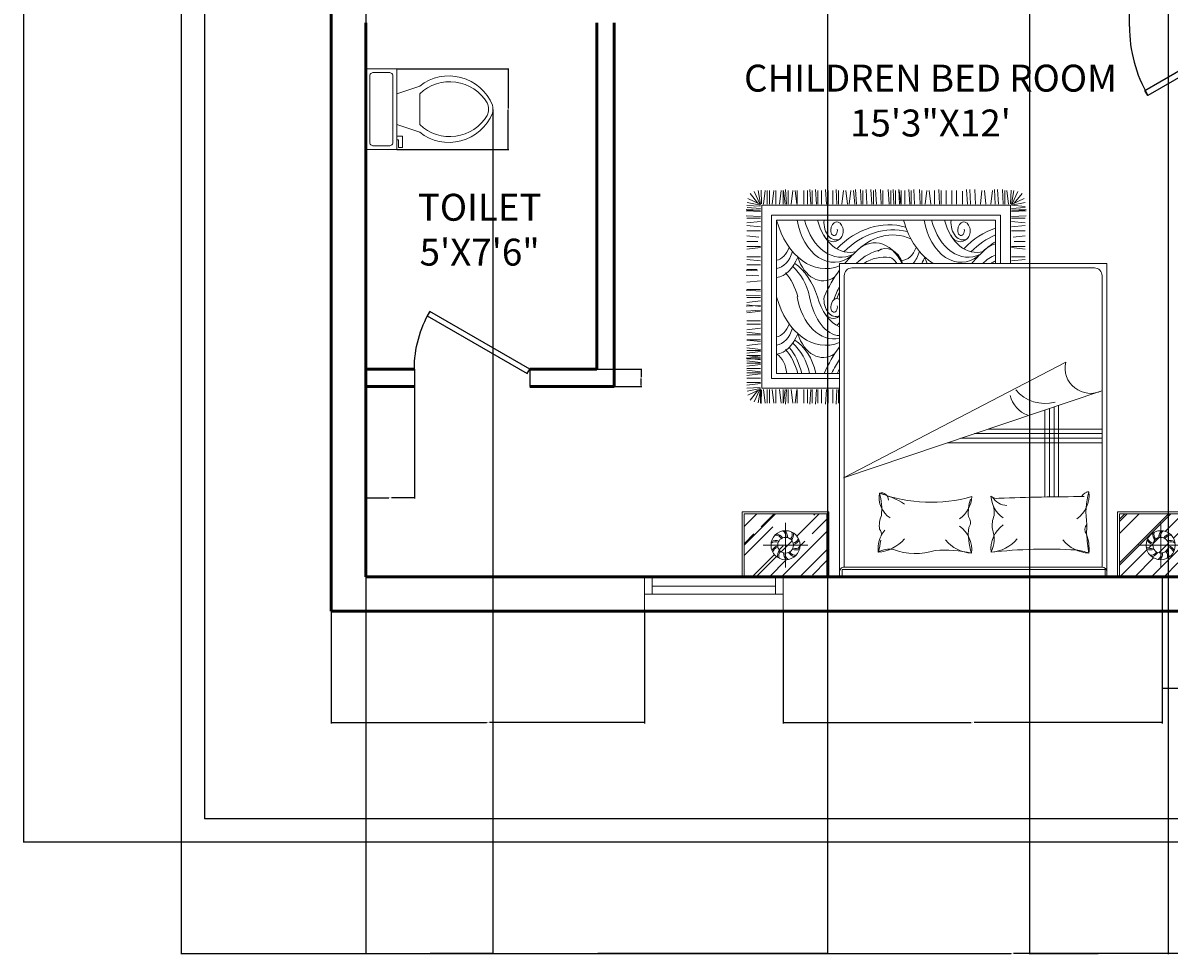
# Model space of a CAD drawing. Units: inches. Extents: x -28 to 483, y -584 to 51.
# Tile 1 of 6: x -28 to 270, y -584 to -342. Entities that reach past the tile are written whole.
import ezdxf

# ---------------------------------------------------------------- set-up
doc = ezdxf.new("R2010")
doc.units = ezdxf.units.IN
doc.header["$MEASUREMENT"] = 0
for name, color, linetype, lineweight in [('A-ANNO-DIMS', 2, 'Continuous', 18), ('A-AREA-IDEN', 7, 'Continuous', 25), ('A-DOOR', 4, 'Continuous', 25), ('A-FLOR-FIXT', 9, 'Continuous', 18), ('A-FURN', 30, 'Continuous', 18), ('A-GLAZ', 5, 'Continuous', 18), ('A-WALL', 7, 'Continuous', 50), ('C-PROP', 7, 'Continuous', 25)]:
    doc.layers.add(name, color=color, linetype=linetype, lineweight=lineweight)
doc.styles.get("Standard").update_dxf_attribs({"font": 'arial.ttf'})
doc.dimstyles.get("Standard").update_dxf_attribs({"dimtxt": 0.18, "dimasz": 0.18, "dimexe": 0.18, "dimexo": 0.0625, "dimgap": 0.09, "dimtad": 0, "dimtih": 1, "dimtoh": 1, "dimdec": 4, "dimzin": 0, "dimdsep": 46, "dimtxsty": 'Standard', "dimcen": 0.09, "dimadec": 0, "dimazin": 0, "dimtfac": 1, "dimtdec": 4, "dimtofl": 0, "dimtmove": 0, "dimatfit": 3, "dimfxl": 1, "dimtolj": 1, "dimtzin": 0, "dimarcsym": 0})

# ---------------------------------------------------------------- blocks, each defined once
blk = doc.blocks.new('*U2')
for p, q in [((0, 0), (0, -6)), ((40, 0), (40, -6))]:
    blk.add_line(p, q)
blk.add_lwpolyline([(0, 0), (34.64, 20), (35.52, 18.48), (0.87, -1.52)], close=True)
blk.add_arc((0, 0), 40, 0, 30)
blk = doc.blocks.new('A$C64B41DC1')
for p, q in [((0, 2.5079), (2.9903, 2.5079)), ((0, 2.0879), (0, 2.5079)), ((0.012, 2.4618), (0.0581, 2.5079)), ((0.012, 2.3515), (0.1684, 2.5079)), ((0.012, 2.0999), (0.012, 2.5079)), ((0.0543, 2.2213), (0.3409, 2.5079)), ((0.1689, 2.4179), (0.2589, 2.5079)), ((0.3265, 2.386), (0.4484, 2.5079)), ((0.3699, 2.3332), (0.5445, 2.5079)), ((0.548, 2.5079), (0.548, 2.0999)), ((0.56, 2.5079), (0.56, 2.0879)), ((0.6301, 2.5079), (0.6301, 0.4779)), ((0.6401, 2.461), (0.6401, 2.5079)), ((0.6401, 2.5079), (2.344, 2.5079)), ((2.344, 2.461), (0.6401, 2.461)), ((2.344, 2.5079), (2.3601, 2.5079)), ((2.344, 2.5079), (2.344, 2.461)), ((2.3601, 2.5079), (2.3601, 2.4761)), ((2.3601, 0.4779), (2.3601, 2.5079)), ((2.4303, 2.5079), (2.4303, 2.0879)), ((2.4423, 2.5079), (2.4423, 2.0999)), ((2.4423, 2.3333), (2.6169, 2.5079)), ((2.4423, 2.2145), (2.7357, 2.5079)), ((2.4423, 2.404), (2.5354, 2.4971)), ((2.705, 2.398), (2.8149, 2.5079)), ((2.7691, 2.3772), (2.8998, 2.5079)), ((2.7819, 2.3646), (2.9252, 2.5079)), ((2.9783, 2.0999), (2.9783, 2.5079)), ((2.9903, 2.0879), (2.9903, 2.5079)), ((0.2157, 2.0999), (0.548, 2.4322)), ((0.2299, 2.0999), (0.548, 2.418)), ((0.2804, 2.1597), (0.2804, 2.4481)), ((0.6601, 2.4461), (1.4951, 2.4461)), ((0.6601, 2.4461), (0.6601, 0.5579)), ((1.4951, 2.4461), (0.6697, 2.4461)), ((2.3301, 2.4461), (1.4951, 2.4461)), ((2.3301, 0.5579), (2.3301, 2.4461)), ((2.7099, 2.1597), (2.7099, 2.4481)), ((0.1362, 2.3039), (0.4246, 2.3039)), ((0.2311, 2.2906), (0.2937, 2.3532)), ((0.3405, 2.3039), (0.3605, 2.3238)), ((2.8541, 2.3039), (2.5657, 2.3039)), ((2.5849, 2.2779), (2.6158, 2.3088)), ((2.6158, 2.3088), (2.6313, 2.3243)), ((2.6674, 2.2756), (2.7382, 2.3464)), ((2.7249, 2.3076), (2.7512, 2.3339)), ((2.7746, 2.0999), (2.9783, 2.3036)), ((2.7914, 2.1846), (2.9783, 2.3715)), ((0.012, 2.261), (0.0275, 2.2765)), ((0.0404, 2.0999), (0.1982, 2.2578)), ((0.2905, 2.2539), (0.3304, 2.2938)), ((0.4194, 2.0999), (0.548, 2.2285)), ((2.4423, 2.1353), (2.5382, 2.2312)), ((2.4918, 2.0999), (2.6366, 2.2447)), ((2.9144, 2.2312), (2.9783, 2.2951)), ((0.1365, 2.0999), (0.251, 2.2144)), ((2.7831, 2.0999), (2.8678, 2.1846)), ((2.8962, 2.0999), (2.9783, 2.182)), ((0.56, 2.0879), (0, 2.0879)), ((0.548, 2.0999), (0.012, 2.0999)), ((0.4986, 2.0999), (0.548, 2.1493)), ((0.5127, 2.0999), (0.548, 2.1352)), ((2.4303, 2.0879), (2.9903, 2.0879)), ((2.4423, 2.0999), (2.9783, 2.0999)), ((2.5172, 2.0999), (2.5269, 2.1096)), ((0.9415, 1.9902), (0.9415, 1.3975)), ((0.9715, 1.9906), (0.9715, 1.4076)), ((1.0015, 1.991), (1.0015, 1.4177)), ((1.0315, 1.9916), (1.0315, 1.4279)), ((2.3349, 1.8678), (0.6613, 1.3029)), ((0.8956, 1.1191), (2.3349, 1.8678)), ((1.6636, 1.6412), (0.6601, 1.6412)), ((1.5748, 1.6112), (0.6601, 1.6112)), ((2.3665, 1.295), (2.3665, 1.3839)), ((2.377, 1.295), (2.3822, 1.3891)), ((2.4032, 1.295), (2.4032, 1.3839)), ((2.4346, 1.295), (2.4346, 1.3839)), ((2.4451, 1.295), (2.4503, 1.3891)), ((2.4774, 1.2957), (2.4774, 1.3837)), ((2.5, 1.295), (2.5, 1.3839)), ((2.5105, 1.295), (2.5157, 1.3891)), ((2.5367, 1.295), (2.5367, 1.3839)), ((2.5471, 1.295), (2.5524, 1.3891)), ((2.5681, 1.295), (2.5681, 1.3839)), ((2.5918, 1.295), (2.5918, 1.3839)), ((2.6346, 1.2957), (2.6346, 1.3837)), ((2.6362, 1.2957), (2.6467, 1.3839)), ((2.6729, 1.295), (2.6624, 1.3839)), ((2.6938, 1.295), (2.6938, 1.3839)), ((2.7043, 1.295), (2.7095, 1.3891)), ((2.7127, 1.2957), (2.7232, 1.3839)), ((2.7253, 1.295), (2.7253, 1.3839)), ((2.7494, 1.295), (2.7389, 1.3839)), ((2.7718, 1.295), (2.7718, 1.3839)), ((2.7959, 1.295), (2.7854, 1.3839)), ((2.8146, 1.2957), (2.8146, 1.3837)), ((2.8146, 1.2957), (2.8146, 1.3837)), ((2.8282, 1.295), (2.8282, 1.3839)), ((2.8282, 1.295), (2.8282, 1.3839)), ((2.8523, 1.295), (2.8418, 1.3839)), ((2.8523, 1.295), (2.8418, 1.3839)), ((2.8653, 1.2966), (2.8688, 1.3861)), ((2.8711, 1.2957), (2.8711, 1.3837)), ((2.8711, 1.2957), (2.8875, 1.3822)), ((2.8765, 1.2958), (2.9132, 1.3758)), ((2.8893, 1.3011), (2.9394, 1.3636)), ((2.3601, 1.2873), (2.8639, 1.2873)), ((2.8639, 1.2873), (2.8639, 0.1018)), ((2.8713, 1.2927), (2.954, 1.3315)), ((2.8716, 1.2565), (2.9605, 1.2669)), ((2.8717, 1.2884), (2.9588, 1.3058)), ((2.8744, 1.2817), (2.9603, 1.2869)), ((2.3601, 1.2233), (2.7999, 1.2233)), ((2.3601, 1.1913), (2.7679, 1.1912)), ((2.7679, 1.1912), (2.7679, 0.1978)), ((2.7999, 1.2233), (2.7999, 0.1658)), ((2.8716, 1.2212), (2.9605, 1.2212)), ((2.8716, 1.1947), (2.9605, 1.2052)), ((2.8723, 1.2489), (2.9603, 1.2489)), ((2.8716, 1.181), (2.9605, 1.1705)), ((2.8716, 1.1595), (2.9605, 1.1595)), ((2.8716, 1.133), (2.9605, 1.1435)), ((2.8716, 1.1193), (2.9605, 1.1088)), ((2.8723, 1.1872), (2.9603, 1.1872)), ((2.8723, 1.1255), (2.9603, 1.1255)), ((2.8716, 1.1035), (2.9605, 1.093)), ((2.8716, 1.0965), (2.9605, 1.0965)), ((2.8716, 1.086), (2.9657, 1.0913)), ((2.8716, 1.0756), (2.9605, 1.0756)), ((2.8716, 1.0491), (2.9605, 1.0596)), ((2.8723, 1.0858), (2.9605, 1.0753)), ((2.8723, 1.0416), (2.9603, 1.0416)), ((2.8716, 1.0354), (2.9605, 1.0249)), ((2.8723, 0.9987), (2.9605, 1.0092)), ((2.8723, 0.985), (2.9605, 0.9745)), ((2.8723, 0.9735), (2.9603, 0.9735)), ((2.8716, 0.9346), (2.9605, 0.9241)), ((2.8723, 0.9408), (2.9603, 0.9408)), ((2.8723, 0.8979), (2.9605, 0.9084)), ((2.8723, 0.8726), (2.9603, 0.8726)), ((2.8723, 0.8505), (2.9603, 0.8505)), ((2.8716, 0.7885), (2.9605, 0.799)), ((2.8716, 0.7818), (2.9657, 0.787)), ((2.8716, 0.7503), (2.9657, 0.7556)), ((2.8723, 0.7571), (2.9605, 0.7466)), ((2.8716, 0.7204), (2.9605, 0.7309)), ((2.8716, 0.6995), (2.9605, 0.6995)), ((2.8716, 0.689), (2.9657, 0.6838)), ((2.8716, 0.6576), (2.9657, 0.6523)), ((2.8716, 0.6471), (2.9605, 0.6471)), ((2.8716, 0.5903), (2.9605, 0.6007)), ((2.882, 0.5582), (2.9657, 0.5536)), ((2.8909, 0.5263), (2.9657, 0.5222)), ((0.6301, 0.4779), (2.3601, 0.4779)), ((0.7101, 0.5079), (2.2801, 0.5079)), ((1.2465, 0.4625), (1.1576, 0.452)), ((1.2542, 0.1018), (1.2542, 0.4779)), ((1.3182, 0.1658), (1.3182, 0.4779)), ((1.3502, 0.1978), (1.3502, 0.4779)), ((2.8716, 0.4877), (2.9603, 0.4877)), ((2.8716, 0.4625), (2.9605, 0.452)), ((2.8928, 0.5169), (2.9605, 0.5169)), ((1.2465, 0.3746), (1.1576, 0.3851)), ((1.2465, 0.4365), (1.1577, 0.4365)), ((2.8716, 0.4365), (2.9603, 0.4365)), ((2.8716, 0.3746), (2.9605, 0.3851)), ((1.2355, 0.3092), (1.1576, 0.3)), ((1.2465, 0.3684), (1.1577, 0.3684)), ((1.2285, 0.3357), (1.1577, 0.3357)), ((2.8716, 0.3684), (2.9603, 0.3684)), ((2.8826, 0.3092), (2.9605, 0.3)), ((2.8896, 0.3357), (2.9603, 0.3357)), ((1.2457, 0.2423), (1.1576, 0.2319)), ((1.2457, 0.2676), (1.1577, 0.2676)), ((2.8723, 0.2676), (2.9603, 0.2676)), ((2.8723, 0.2423), (2.9605, 0.2319)), ((1.2465, 0.1742), (1.1524, 0.169)), ((1.2465, 0.2057), (1.1576, 0.2161)), ((1.2465, 0.1847), (1.1576, 0.1847)), ((2.7999, 0.1658), (1.3182, 0.1658)), ((2.7679, 0.1978), (1.3502, 0.1978)), ((2.8716, 0.2057), (2.9605, 0.2161)), ((2.8716, 0.1847), (2.9605, 0.1847)), ((2.8716, 0.1742), (2.9657, 0.169)), ((1.2465, 0.1428), (1.1524, 0.1376)), ((1.2465, 0.1334), (1.1524, 0.1281)), ((1.2465, 0.1323), (1.1576, 0.1323)), ((1.2465, 0.1323), (1.1576, 0.1323)), ((1.2465, 0.1), (1.1576, 0.1105)), ((1.2465, 0.1229), (1.1588, 0.1168)), ((1.2464, 0.1007), (1.1592, 0.0833)), ((1.2468, 0.0964), (1.1641, 0.0576)), ((1.2288, 0.088), (1.1787, 0.0255)), ((1.2415, 0.0933), (1.2049, 0.0133)), ((1.247, 0.0934), (1.2306, 0.0069)), ((1.2527, 0.0925), (1.2493, 0.003)), ((2.8639, 0.1018), (1.2542, 0.1018)), ((1.2658, 0.0941), (1.2762, 0.0052)), ((1.2899, 0.0941), (1.2899, 0.0052)), ((1.2999, 0.0941), (1.3051, 0)), ((1.3313, 0.0941), (1.3365, 0)), ((1.3523, 0.0941), (1.3575, 0)), ((1.3804, 0.0941), (1.3699, 0.0052)), ((1.4119, 0.0934), (1.4223, 0.0052)), ((1.4485, 0.0941), (1.438, 0.0052)), ((1.48, 0.0941), (1.4852, 0)), ((1.5114, 0.0941), (1.5166, 0)), ((1.5323, 0.0941), (1.5376, 0)), ((1.5638, 0.0941), (1.5638, 0.0105)), ((1.6021, 0.0941), (1.6021, 0.0052)), ((1.6336, 0.0941), (1.6336, 0.0052)), ((1.6702, 0.0941), (1.6702, 0.0052)), ((1.7017, 0.0941), (1.7017, 0.0052)), ((1.7122, 0.0941), (1.7174, 0)), ((1.7445, 0.0934), (1.7445, 0.0054)), ((1.7698, 0.0934), (1.7803, 0.0052)), ((1.8065, 0.0941), (1.796, 0.0052)), ((1.8274, 0.0941), (1.8274, 0.0052)), ((1.8379, 0.0941), (1.8431, 0)), ((1.8746, 0.0941), (1.8798, 0)), ((1.8955, 0.0941), (1.8955, 0.0052)), ((1.906, 0.0941), (1.9113, 0)), ((1.9384, 0.0934), (1.9384, 0.0054)), ((1.9609, 0.0941), (1.9609, 0.0052)), ((1.9636, 0.0934), (1.9741, 0.0052)), ((1.9714, 0.0941), (1.9766, 0)), ((1.9976, 0.0941), (1.9976, 0.0052)), ((2.0081, 0.0941), (2.0133, 0)), ((2.029, 0.0941), (2.029, 0.0052)), ((2.0395, 0.0941), (2.0447, 0)), ((2.0797, 0.0941), (2.0797, 0.0052)), ((2.0902, 0.0941), (2.0954, 0)), ((2.1216, 0.0941), (2.1269, 0)), ((2.1412, 0.0941), (2.1412, 0.0052)), ((2.1517, 0.0941), (2.1569, 0)), ((2.1831, 0.0941), (2.1884, 0)), ((2.2093, 0.0941), (2.2093, 0.0052)), ((2.2198, 0.0941), (2.225, 0)), ((2.2512, 0.0941), (2.2565, 0)), ((2.2603, 0.0934), (2.2707, 0.0052)), ((2.2969, 0.0941), (2.2864, 0.0052)), ((2.3089, 0.0934), (2.3193, 0.0052)), ((2.3455, 0.0941), (2.3351, 0.0052)), ((2.3665, 0.0941), (2.3665, 0.0052)), ((2.377, 0.0941), (2.3822, 0)), ((2.4032, 0.0941), (2.4032, 0.0052)), ((2.4346, 0.0941), (2.4346, 0.0052)), ((2.4451, 0.0941), (2.4503, 0)), ((2.4774, 0.0934), (2.4774, 0.0054)), ((2.5, 0.0941), (2.5, 0.0052)), ((2.5105, 0.0941), (2.5157, 0)), ((2.5367, 0.0941), (2.5367, 0.0052)), ((2.5471, 0.0941), (2.5524, 0)), ((2.5681, 0.0941), (2.5681, 0.0052)), ((2.5918, 0.0941), (2.5918, 0.0052)), ((2.6346, 0.0934), (2.6346, 0.0054)), ((2.6362, 0.0934), (2.6467, 0.0052)), ((2.6729, 0.0941), (2.6624, 0.0052)), ((2.6938, 0.0941), (2.6938, 0.0052)), ((2.7043, 0.0941), (2.7095, 0)), ((2.7127, 0.0934), (2.7232, 0.0052)), ((2.7253, 0.0941), (2.7253, 0.0052)), ((2.7494, 0.0941), (2.7389, 0.0052)), ((2.7718, 0.0941), (2.7718, 0.0052)), ((2.7959, 0.0941), (2.7854, 0.0052)), ((2.8146, 0.0934), (2.8146, 0.0054)), ((2.8282, 0.0941), (2.8282, 0.0052)), ((2.8523, 0.0941), (2.8418, 0.0052)), ((2.8653, 0.0925), (2.8688, 0.003)), ((2.8711, 0.0934), (2.8875, 0.0069)), ((2.8713, 0.0964), (2.954, 0.0576)), ((2.8716, 0.1428), (2.9657, 0.1376)), ((2.8716, 0.1334), (2.9657, 0.1281)), ((2.8716, 0.1323), (2.9605, 0.1323)), ((2.8716, 0.1229), (2.9593, 0.1168)), ((2.8717, 0.1007), (2.9588, 0.0833)), ((2.8744, 0.1074), (2.9603, 0.1022)), ((2.8765, 0.0933), (2.9132, 0.0133)), ((2.8893, 0.088), (2.9394, 0.0255))]:
    blk.add_line(p, q)
at = {"ltscale": 10}
for p, q in [((1.4859, 1.5812), (0.6601, 1.5812)), ((1.397, 1.5512), (0.6601, 1.5512))]:
    blk.add_line(p, q, dxfattribs=at)
for centre, radius in [((0.2804, 2.3039), 0.0942), ((2.7099, 2.3039), 0.0942), ((0.2804, 2.3039), 0.051), ((2.7099, 2.3039), 0.051)]:
    blk.add_circle(centre, radius)
for centre, radius, start, end in [((0.6601, 2.4761), 0.03, 180, 270), ((2.3301, 2.4761), 0.03, 270, 0), ((0.2887, 2.3745), 0.0605, 172.17003, 218.48975), ((0.2828, 2.3731), 0.0462, 160.30017, 220.53802), ((0.3286, 2.3561), 0.0605, 136.17003, 182.48975), ((0.3231, 2.3585), 0.0462, 124.30017, 184.53802), ((0.3501, 2.3178), 0.0605, 100.17003, 146.48975), ((2.6402, 2.3178), 0.0605, 33.51025, 79.82997), ((2.6672, 2.3585), 0.0462, 355.46198, 55.69983), ((2.6617, 2.3561), 0.0605, 357.51025, 43.82997), ((2.7075, 2.3731), 0.0462, 319.46198, 19.69983), ((2.7016, 2.3745), 0.0605, 321.51025, 7.82997), ((0.2457, 2.3659), 0.0605, 208.17003, 254.48975), ((0.2417, 2.3614), 0.0462, 196.30017, 256.53802), ((0.347, 2.323), 0.0462, 88.30017, 148.53802), ((0.3449, 2.2742), 0.0605, 64.17003, 110.48975), ((0.3455, 2.2802), 0.0462, 52.30017, 112.53802), ((1.0526, 2.3302), 0.3085, 175.30484, 198.69419), ((-0.8702, 2.0941), 1.6364, 4.80985, 9.18918), ((0.8579, 2.6278), 0.2948, 247.51785, 264.26696), ((0.728, 2.111), 0.245, 40.4189, 85.9871), ((1.0164, 5.7096), 3.3803, 266.81337, 276.16021), ((1.3963, 2.1044), 0.245, 94.0129, 139.5811), ((1.1858, 2.3288), 0.1943, 306.5711, 5.88998), ((1.5348, 2.2652), 0.1767, 151.77364, 201.69827), ((1.6986, 2.3355), 0.1943, 174.11002, 233.4289), ((1.1481, 2.2311), 0.3783, 353.49469, 19.18669), ((1.6871, 3.192), 0.8561, 257.74383, 273.62843), ((1.4882, 2.111), 0.245, 40.4189, 85.9871), ((1.8674, 1.9709), 0.3878, 68.20259, 108.9817), ((2.1269, 2.1044), 0.245, 94.0129, 139.5811), ((2.0342, 2.4856), 0.1563, 261.59582, 298.90918), ((1.9165, 2.3288), 0.1943, 333.73715, 5.88998), ((2.6058, 2.2028), 0.517, 163.60457, 172.3273), ((2.6448, 2.2802), 0.0462, 67.46198, 127.69983), ((2.6454, 2.2742), 0.0605, 69.51025, 115.82997), ((2.6433, 2.323), 0.0462, 31.46198, 91.69983), ((2.7486, 2.3614), 0.0462, 283.46198, 343.69983), ((2.7446, 2.3659), 0.0605, 285.51025, 331.82997), ((0.2153, 2.3276), 0.0462, 232.30017, 292.53802), ((0.2158, 2.3336), 0.0605, 244.17003, 290.48975), ((0.2138, 2.2848), 0.0462, 268.30017, 328.53802), ((0.2107, 2.29), 0.0605, 280.17003, 326.48975), ((0.2377, 2.2493), 0.0462, 304.30017, 4.53802), ((0.2322, 2.2517), 0.0605, 316.17003, 2.48975), ((0.2779, 2.2347), 0.0462, 340.30017, 40.53802), ((0.272, 2.2333), 0.0605, 352.17003, 38.48975), ((0.3191, 2.2464), 0.0462, 16.30017, 76.53802), ((0.3151, 2.2419), 0.0605, 28.17003, 74.48975), ((0.7274, 2.2013), 0.0446, 314.4736, 42.17134), ((-1.6008, 2.277), 2.3618, 357.39054, 358.88764), ((1.9165, 2.3288), 0.1943, 320.94042, 333.73715), ((2.1347, 2.2313), 0.0459, 165.35061, 223.26844), ((2.6752, 2.2419), 0.0605, 105.51025, 151.82997), ((2.6712, 2.2464), 0.0462, 103.46198, 163.69983), ((2.7182, 2.2333), 0.0605, 141.51025, 187.82997), ((2.7123, 2.2347), 0.0462, 139.46198, 199.69983), ((2.7581, 2.2517), 0.0605, 177.51025, 223.82997), ((2.7526, 2.2493), 0.0462, 175.46198, 235.69983), ((2.7796, 2.29), 0.0605, 213.51025, 259.82997), ((2.7765, 2.2848), 0.0462, 211.46198, 271.69983), ((2.7744, 2.3336), 0.0605, 249.51025, 295.82997), ((2.775, 2.3276), 0.0462, 247.46198, 307.69983), ((0.2688, 2.0945), 0.4956, 344.0243, 8.70709), ((1.204, 2.1778), 0.1681, 337.01697, 7.53676), ((1.5671, 2.1546), 0.0547, 142.08329, 220.902), ((1.9346, 2.1778), 0.1681, 337.01697, 7.53676), ((0.9385, 1.978), 0.1943, 126.5711, 185.88998), ((1.1858, 1.9714), 0.1943, 4.31813, 53.4289), ((1.5415, 2.0969), 0.1834, 175.22328, 196.23004), ((1.7059, 1.9714), 0.204, 127.11975, 175.09005), ((1.1965, 2.0983), 0.3299, 343.79543, 3.55541), ((1.9394, 1.991), 0.1651, 351.26213, 55.75721), ((2.4617, 2.0719), 0.3745, 173.82958, 196.4356), ((1.2687, 1.9248), 0.1223, 33.62799, 86.47438), ((1.7676, 1.0629), 0.9631, 69.65065, 105.96307), ((2.2748, 2.5795), 0.6373, 238.34989, 254.31375), ((2.0911, 2.0123), 0.0478, 179.77267, 283.80184), ((0.7417, 2.0149), 0.057, 273.47085, 328.54118), ((0.728, 2.2025), 0.245, 274.0129, 278.34166), ((0.7246, 18.8439), 16.8552, 270.17399, 272.05214), ((1.3401, 1.9404), 0.0603, 49.09906, 101.37023), ((1.0747, 1.2871), 0.1871, 14.1863, 69.12121), ((1.0274, 1.1334), 0.2527, 40.62904, 104.37123), ((0.7347, 1.1553), 0.1649, 347.31088, 116.44537), ((0.7101, 0.5579), 0.05, 180, 270), ((2.2801, 0.5579), 0.05, 270, 0)]:
    blk.add_arc(centre, radius, start, end)
for centre, major_axis, ratio, start_param, end_param in [((1.9938, 1.6262), (0, -0.7531), 0.68, 0.797284, 0.954936), ((2.0643, 1.466), (0, -0.5322), 0.68, 7.239912, 7.311536), ((1.9052, 1.7397), (0, -0.9842), 0.68, 0.74745, 0.979724), ((2.7455, 1.3081), (0, 0.3614), 0.68, 1.900046, 2.742661), ((2.7868, 1.3081), (0, 0.3614), 0.68, 1.900046, 2.614747), ((2.8372, 1.3081), (0, 0.3614), 0.68, 1.900046, 2.479658), ((2.8607, 1.3211), (0, 0.3614), 0.68, 1.938265, 2.479658), ((2.8057, 1.2079), (0, -0.1524), 0.68, 4.821745, 5.895886), ((2.4665, 0.8216), (0, -0.2664), 0.68, 2.006169, 3.565187), ((2.4513, 0.5069), (0, 0.502), 0.68, 5.095327, 6.553458), ((2.7862, 0.8069), (0, -0.2615), 0.68, 3.244645, 4.205018), ((2.396, 0.6032), (0, 0.3641), 0.68, -1.3172, 0.145284), ((2.7784, 0.8289), (0, -0.1802), 0.68, 3.227058, 4.318474), ((2.3507, 0.5642), (0.0073, 0.3819), 0.56205, -1.21172, -0.009991), ((2.7821, 0.7971), (0, -0.1589), 0.68, 3.272942, 4.229533), ((2.2964, 0.5771), (0, -0.3263), 0.68, 1.938944, 2.850232), ((2.0403, 1.6015), (0, -0.8763), 0.68, 6.849801, 6.887077), ((2.4005, 0.7132), (0, -0.1214), 0.68, 2.284368, 3.652258), ((2.3834, 0.7081), (0, 0.1147), 0.68, 4.593909, 6.585576), ((2.3774, 0.7653), (0, -0.0593), 0.68, 5.841311, 7.755362), ((2.3961, 0.7628), (0, -0.0317), 0.68, 1.462497, 5.046281), ((1.9938, 1.1295), (-0.0678, 0.7439), 0.610498, 3.917146, 4.063997), ((2.0643, 0.9693), (0, -0.5322), 0.68, 7.239912, 7.336618), ((1.9052, 1.243), (0, -0.9842), 0.68, 0.74745, 0.979724), ((2.7455, 0.8114), (-0.0599, 0.3735), 0.695517, 1.775813, 2.548612), ((2.7868, 0.8114), (0, 0.3614), 0.68, 1.900046, 2.614747), ((2.8607, 0.8243), (0, 0.3614), 0.68, 1.938265, 2.479658), ((2.4665, 0.3249), (0, -0.2664), 0.68, 2.006169, 3.565187), ((2.4513, 0.0102), (0, 0.502), 0.68, 5.095327, 6.553458), ((2.7862, 0.3102), (0, -0.2615), 0.68, 3.244645, 4.205018), ((1.242, 0.9693), (0, -0.5322), 0.68, 6.586764, 6.677612), ((1.1714, 1.1295), (-0.1157, 0.7241), 0.59432, 3.291697, 3.50733), ((1.0828, 1.243), (0, -0.9842), 0.68, 0.565948, 0.680366), ((1.5283, 0.0674), (0, -0.3703), 0.68, 1.930561, 3.464283), ((1.5736, 0.1065), (0, 0.3641), 0.68, -1.3172, 0.476403), ((1.6289, 0.0102), (0, 0.502), 0.68, 6.655152, 6.661293), ((1.6289, 0.0102), (0, 0.502), 0.68, 5.095327, 5.911219), ((1.6442, 0.3249), (0, -0.2664), 0.68, 2.006169, 2.182797), ((1.9638, 0.3102), (0, -0.2615), 0.68, 4.015924, 4.205018), ((1.956, 0.3322), (0, -0.1802), 0.68, 3.770744, 4.318474), ((1.9597, 0.3004), (0, -0.1589), 0.68, 3.14258, 4.229533), ((2.0606, 0.5616), (0, -0.1803), 0.68, 5.194792, 5.929328), ((2.0606, 0.5616), (0, -0.1803), 0.68, 5.194792, 6.723255), ((2.1315, 0.6603), (0, -0.3155), 0.68, 5.328638, 6.949396), ((2.0549, 0.5656), (0, -0.1303), 0.68, 5.450951, 6.054641), ((2.0643, 0.9693), (0, -0.5322), 0.68, 6.20013, 6.677612), ((1.9938, 1.1295), (-0.0678, 0.7439), 0.610498, 3.199135, 3.592282), ((1.9052, 1.243), (0, -0.9842), 0.68, 0.565948, 0.680366), ((2.3507, 0.0674), (0, -0.3703), 0.68, 1.930561, 3.464283), ((2.396, 0.1065), (0, 0.3641), 0.68, -1.3172, 0.476403), ((2.4513, 0.0102), (0, 0.502), 0.68, 6.655152, 6.661293), ((2.7784, 0.3322), (0, -0.1802), 0.68, 3.227058, 4.318474), ((2.7821, 0.3004), (0, -0.1589), 0.68, 3.272942, 4.229533), ((1.1933, 0.9181), (0, -0.624), 0.68, 0.378672, 0.625379), ((1.3091, 0.6603), (0, -0.3155), 0.68, 6.475719, 6.949396), ((1.1911, 1.1066), (0, 0.8458), 0.68, 3.421828, 3.728616), ((1.2179, 1.1047), (0, -0.8763), 0.68, 6.507006, 6.887077), ((1.474, 0.0804), (0, -0.3263), 0.68, 1.938944, 3.339184), ((2.0157, 0.9181), (0, -0.624), 0.68, -0.280078, 0.625379), ((2.0135, 1.1066), (0, 0.8458), 0.68, 2.978727, 3.728616), ((2.0403, 1.1047), (0, -0.8763), 0.68, 6.099302, 6.887077), ((2.2964, 0.0804), (0, -0.3263), 0.68, 1.938944, 3.339184), ((1.555, 0.2685), (0, -0.0593), 0.68, 3.732151, 7.755362), ((1.5781, 0.2165), (0, -0.1214), 0.68, 2.284368, 3.726131), ((1.561, 0.2114), (0, 0.1147), 0.68, 4.593909, 6.647252), ((1.5737, 0.2661), (0, -0.0317), 0.68, 1.462497, 5.046281), ((2.3774, 0.2685), (0, -0.0593), 0.68, 3.732151, 7.755362), ((2.4005, 0.2165), (0, -0.1214), 0.68, 2.284368, 3.726131), ((2.3834, 0.2114), (0, 0.1147), 0.68, 4.593909, 6.647252), ((2.3961, 0.2661), (0, -0.0317), 0.68, 1.462497, 5.046281)]:
    blk.add_ellipse(centre, major_axis=major_axis, ratio=ratio, start_param=start_param, end_param=end_param)
blk = doc.blocks.new('*U5')
for p, q in [((9.5, -6), (9.5, -2)), ((-10, -8.5), (-8, -8.5)), ((-10, -9.5), (-10, -8.5)), ((-8, -8.5), (-8, -8)), ((-7, -8), (-7, -9.5)), ((-4, -8), (-6, -14)), ((4, -8), (6, -14)), ((-7, -9.5), (-10, -9.5)), ((4, -14), (-4, -14))]:
    blk.add_line(p, q)
blk.add_lwpolyline([(10.5, -8), (10.5, 0), (-10.5, 0), (-10.5, -8)], close=True)
for points in [[(-9.5, -2), (-9.5, -6)], [(8.5, -1), (-8.5, -1)], [(-8.5, -7), (8.5, -7)]]:
    blk.add_lwpolyline(points)
for centre, radius, start, end in [((-8.62, -1.88), 0.884, 81.8699, 188.1301), ((8.62, -1.88), 0.884, 351.8699, 98.1301), ((-8.62, -6.12), 0.884, 171.8699, 278.1301), ((8.62, -6.12), 0.884, 261.8699, 8.1301), ((3.52, -21.58), 12.17, 141.4691, 247.9714), ((4.2, -21.82), 11.33, 136.3677, 238.9468), ((-3.52, -21.58), 12.17, 292.0284, 38.5307), ((-4.2, -21.82), 11.33, 301.053, 43.6321), ((0, -27.88), 4, 245.7318, 294.2682), ((0, -29), 4, 254.8605, 285.1395)]:
    blk.add_arc(centre, radius, start, end)
blk = doc.blocks.new('WIN-36IN')
for p, q in [((0, 9), (0, 0)), ((2, 9), (2, 4.5)), ((34, 9), (34, 4.5)), ((36, 9), (36, 0)), ((34, 6.5), (2, 6.5)), ((36, 4.5), (0, 4.5))]:
    blk.add_line(p, q)
blk = doc.blocks.new('*D19')
at = {"layer": 'A-ANNO-DIMS', "color": 0, "lineweight": -2, "transparency": 16777216}
for p, q in [((12.84, -554.65), (12.84, -583.72)), ((444.84, -554.65), (444.84, -583.72)), ((13.02, -583.54), (228.55, -583.54)), ((444.66, -583.54), (229.13, -583.54))]:
    blk.add_line(p, q, dxfattribs=at)
at = {"layer": 'A-ANNO-DIMS', "color": 0, "transparency": 16777216}
for points in [[(13.02, -583.51), (13.02, -583.57), (12.84, -583.54)], [(444.66, -583.51), (444.66, -583.57), (444.84, -583.54)]]:
    blk.add_solid(points, dxfattribs=at)
at = {"layer": 'Defpoints', "color": 0, "transparency": 16777216}
for p in [(12.84, -554.59), (444.84, -554.59), (444.84, -583.54)]:
    blk.add_point(p, dxfattribs=at)
at = {"layer": 'A-ANNO-DIMS', "color": 0, "transparency": 16777216, "insert": (228.84, -583.54), "char_height": 0.18, "attachment_point": 5}
blk.add_mtext('\\A1;432', dxfattribs=at)
blk = doc.blocks.new('*D20')
at = {"layer": 'A-ANNO-DIMS', "color": 0, "lineweight": -2, "transparency": 16777216}
for p, q in [((12.78, 21.41), (-28.29, 21.41)), ((-28.11, 21.23), (-28.11, -266.41)), ((-28.11, -554.41), (-28.11, -266.77)), ((12.78, -554.59), (-28.29, -554.59))]:
    blk.add_line(p, q, dxfattribs=at)
at = {"layer": 'A-ANNO-DIMS', "color": 0, "transparency": 16777216}
for points in [[(-28.14, 21.23), (-28.08, 21.23), (-28.11, 21.41)], [(-28.14, -554.41), (-28.08, -554.41), (-28.11, -554.59)]]:
    blk.add_solid(points, dxfattribs=at)
at = {"layer": 'Defpoints', "color": 0, "transparency": 16777216}
for p in [(-28.11, 21.41), (12.84, 21.41), (12.84, -554.59)]:
    blk.add_point(p, dxfattribs=at)
at = {"layer": 'A-ANNO-DIMS', "color": 0, "transparency": 16777216, "insert": (-28.11, -266.59), "char_height": 0.18, "attachment_point": 5}
blk.add_mtext('\\A1;576', dxfattribs=at)
blk = doc.blocks.new('*D26')
at = {"layer": 'A-ANNO-DIMS', "color": 0, "lineweight": -2, "transparency": 16777216}
for p, q in [((60.84, -337.15), (60.84, -583.72)), ((180.84, -337.15), (180.84, -583.72)), ((61.02, -583.54), (120.56, -583.54)), ((180.66, -583.54), (121.12, -583.54))]:
    blk.add_line(p, q, dxfattribs=at)
at = {"layer": 'A-ANNO-DIMS', "color": 0, "transparency": 16777216}
for points in [[(61.02, -583.51), (61.02, -583.57), (60.84, -583.54)], [(180.66, -583.51), (180.66, -583.57), (180.84, -583.54)]]:
    blk.add_solid(points, dxfattribs=at)
at = {"layer": 'Defpoints', "color": 0, "transparency": 16777216}
for p in [(60.84, -337.09), (180.84, -337.09), (180.84, -583.54)]:
    blk.add_point(p, dxfattribs=at)
at = {"layer": 'A-ANNO-DIMS', "color": 0, "transparency": 16777216, "insert": (120.84, -583.54), "char_height": 0.18, "attachment_point": 5}
blk.add_mtext('\\A1;120', dxfattribs=at)
blk = doc.blocks.new('*D28')
at = {"layer": 'A-ANNO-DIMS', "color": 0, "lineweight": -2, "transparency": 16777216}
for p, q in [((233.35, -193.15), (233.35, -583.72)), ((269.35, -193.15), (269.35, -583.72)), ((233.53, -583.54), (251.13, -583.54)), ((269.17, -583.54), (251.57, -583.54))]:
    blk.add_line(p, q, dxfattribs=at)
at = {"layer": 'A-ANNO-DIMS', "color": 0, "transparency": 16777216}
for points in [[(233.53, -583.51), (233.53, -583.57), (233.35, -583.54)], [(269.17, -583.51), (269.17, -583.57), (269.35, -583.54)]]:
    blk.add_solid(points, dxfattribs=at)
at = {"layer": 'Defpoints', "color": 0, "transparency": 16777216}
for p in [(233.35, -193.09), (269.35, -193.09), (269.35, -583.54)]:
    blk.add_point(p, dxfattribs=at)
at = {"layer": 'A-ANNO-DIMS', "color": 0, "transparency": 16777216, "insert": (251.35, -583.54), "char_height": 0.18, "attachment_point": 5}
blk.add_mtext('\\A1;36', dxfattribs=at)
blk = doc.blocks.new('*D36')
at = {"layer": 'A-ANNO-DIMS', "color": 0, "lineweight": -2, "transparency": 16777216}
for p, q in [((51.84, -494.65), (51.84, -523.72)), ((133.26, -494.65), (133.26, -523.72)), ((52.02, -523.54), (92.17, -523.54)), ((133.08, -523.54), (92.93, -523.54))]:
    blk.add_line(p, q, dxfattribs=at)
at = {"layer": 'A-ANNO-DIMS', "color": 0, "transparency": 16777216}
for points in [[(52.02, -523.51), (52.02, -523.57), (51.84, -523.54)], [(133.08, -523.51), (133.08, -523.57), (133.26, -523.54)]]:
    blk.add_solid(points, dxfattribs=at)
at = {"layer": 'Defpoints', "color": 0, "transparency": 16777216}
for p in [(51.84, -494.59), (133.26, -494.59), (51.84, -523.54)]:
    blk.add_point(p, dxfattribs=at)
at = {"layer": 'A-ANNO-DIMS', "color": 0, "transparency": 16777216, "insert": (92.55, -523.54), "char_height": 0.18, "attachment_point": 5}
blk.add_mtext('\\A1;81.41', dxfattribs=at)
blk = doc.blocks.new('*D39')
at = {"layer": 'A-ANNO-DIMS', "color": 0, "lineweight": -2, "transparency": 16777216}
for p, q in [((93.84, -364.08), (93.84, -583.72)), ((60.84, -374.58), (60.84, -583.72)), ((61.02, -583.54), (77.12, -583.54)), ((93.66, -583.54), (77.56, -583.54))]:
    blk.add_line(p, q, dxfattribs=at)
at = {"layer": 'A-ANNO-DIMS', "color": 0, "transparency": 16777216}
for points in [[(61.02, -583.51), (61.02, -583.57), (60.84, -583.54)], [(93.66, -583.51), (93.66, -583.57), (93.84, -583.54)]]:
    blk.add_solid(points, dxfattribs=at)
at = {"layer": 'Defpoints', "color": 0, "transparency": 16777216}
for p in [(93.84, -364.02), (60.84, -374.52), (93.84, -583.54)]:
    blk.add_point(p, dxfattribs=at)
at = {"layer": 'A-ANNO-DIMS', "color": 0, "transparency": 16777216, "insert": (77.34, -583.54), "char_height": 0.18, "attachment_point": 5}
blk.add_mtext('\\A1;33', dxfattribs=at)
blk = doc.blocks.new('*D40')
at = {"layer": 'A-ANNO-DIMS', "color": 0, "lineweight": -2, "transparency": 16777216}
for p, q in [((68.91, -353.52), (97.97, -353.52)), ((97.79, -353.7), (97.79, -363.84)), ((97.79, -374.34), (97.79, -364.2)), ((68.91, -374.52), (97.97, -374.52))]:
    blk.add_line(p, q, dxfattribs=at)
at = {"layer": 'A-ANNO-DIMS', "color": 0, "transparency": 16777216}
for points in [[(97.76, -353.7), (97.82, -353.7), (97.79, -353.52)], [(97.76, -374.34), (97.82, -374.34), (97.79, -374.52)]]:
    blk.add_solid(points, dxfattribs=at)
at = {"layer": 'Defpoints', "color": 0, "transparency": 16777216}
for p in [(68.84, -353.52), (68.84, -374.52), (97.79, -374.52)]:
    blk.add_point(p, dxfattribs=at)
at = {"layer": 'A-ANNO-DIMS', "color": 0, "transparency": 16777216, "insert": (97.79, -364.02), "char_height": 0.18, "attachment_point": 5}
blk.add_mtext('\\A1;21', dxfattribs=at)
blk = doc.blocks.new('*D42')
at = {"layer": 'A-ANNO-DIMS', "color": 0, "lineweight": -2, "transparency": 16777216}
for p, q in [((169.26, -494.65), (169.26, -523.72)), ((267.84, -494.65), (267.84, -523.72)), ((169.44, -523.54), (218.16, -523.54)), ((267.66, -523.54), (218.94, -523.54))]:
    blk.add_line(p, q, dxfattribs=at)
at = {"layer": 'A-ANNO-DIMS', "color": 0, "transparency": 16777216}
for points in [[(169.44, -523.51), (169.44, -523.57), (169.26, -523.54)], [(267.66, -523.51), (267.66, -523.57), (267.84, -523.54)]]:
    blk.add_solid(points, dxfattribs=at)
at = {"layer": 'Defpoints', "color": 0, "transparency": 16777216}
for p in [(169.26, -494.59), (267.84, -494.59), (169.26, -523.54)]:
    blk.add_point(p, dxfattribs=at)
at = {"layer": 'A-ANNO-DIMS', "color": 0, "transparency": 16777216, "insert": (218.55, -523.54), "char_height": 0.18, "attachment_point": 5}
blk.add_mtext('\\A1;98.59', dxfattribs=at)
blk = doc.blocks.new('*D43')
at = {"layer": 'A-ANNO-DIMS', "color": 0, "lineweight": -2, "transparency": 16777216}
for p, q in [((267.84, -485.65), (267.84, -514.72)), ((299.34, -485.65), (299.34, -514.72)), ((268.02, -514.54), (283.27, -514.54)), ((299.16, -514.54), (283.92, -514.54))]:
    blk.add_line(p, q, dxfattribs=at)
at = {"layer": 'A-ANNO-DIMS', "color": 0, "transparency": 16777216}
for points in [[(268.02, -514.51), (268.02, -514.57), (267.84, -514.54)], [(299.16, -514.51), (299.16, -514.57), (299.34, -514.54)]]:
    blk.add_solid(points, dxfattribs=at)
at = {"layer": 'Defpoints', "color": 0, "transparency": 16777216}
for p in [(267.84, -485.59), (299.34, -485.59), (267.84, -514.54)]:
    blk.add_point(p, dxfattribs=at)
at = {"layer": 'A-ANNO-DIMS', "color": 0, "transparency": 16777216, "insert": (283.59, -514.54), "char_height": 0.18, "attachment_point": 5}
blk.add_mtext('\\A1;31.5', dxfattribs=at)
blk = doc.blocks.new('*D45')
at = {"layer": 'A-ANNO-DIMS', "color": 0, "lineweight": -2, "transparency": 16777216}
for p, q in [((103.51, -431.59), (132.57, -431.59)), ((132.39, -431.77), (132.39, -433.66)), ((132.39, -435.91), (132.39, -434.02)), ((103.51, -436.09), (132.57, -436.09))]:
    blk.add_line(p, q, dxfattribs=at)
at = {"layer": 'A-ANNO-DIMS', "color": 0, "transparency": 16777216}
for points in [[(132.36, -431.77), (132.42, -431.77), (132.39, -431.59)], [(132.36, -435.91), (132.42, -435.91), (132.39, -436.09)]]:
    blk.add_solid(points, dxfattribs=at)
at = {"layer": 'Defpoints', "color": 0, "transparency": 16777216}
for p in [(103.44, -431.59), (103.44, -436.09), (132.39, -436.09)]:
    blk.add_point(p, dxfattribs=at)
at = {"layer": 'A-ANNO-DIMS', "color": 0, "transparency": 16777216, "insert": (132.39, -433.84), "char_height": 0.18, "attachment_point": 5}
blk.add_mtext('\\A1;4.5', dxfattribs=at)
blk = doc.blocks.new('*D47')
at = {"layer": 'A-ANNO-DIMS', "color": 0, "lineweight": -2, "transparency": 16777216}
for p, q in [((60.84, -436.15), (60.84, -465.22)), ((73.44, -436.15), (73.44, -465.22)), ((61.02, -465.04), (66.83, -465.04)), ((73.26, -465.04), (67.46, -465.04))]:
    blk.add_line(p, q, dxfattribs=at)
at = {"layer": 'A-ANNO-DIMS', "color": 0, "transparency": 16777216}
for points in [[(61.02, -465.01), (61.02, -465.07), (60.84, -465.04)], [(73.26, -465.01), (73.26, -465.07), (73.44, -465.04)]]:
    blk.add_solid(points, dxfattribs=at)
at = {"layer": 'Defpoints', "color": 0, "transparency": 16777216}
for p in [(60.84, -436.09), (73.44, -436.09), (60.84, -465.04)]:
    blk.add_point(p, dxfattribs=at)
at = {"layer": 'A-ANNO-DIMS', "color": 0, "transparency": 16777216, "insert": (67.14, -465.04), "char_height": 0.18, "attachment_point": 5}
blk.add_mtext('\\A1;12.6', dxfattribs=at)

msp = doc.modelspace()

# ---------------------------------------------------------------- linework, layer by layer
at = {"layer": 'A-GLAZ'}
msp.add_line((267.8432, -485.5877), (267.8432, -494.5877), dxfattribs=at)
at = {"layer": 'A-WALL'}
for p, q in [((51.8432, -17.5877), (51.8432, -494.5877)), ((60.8432, -341.5877), (60.8432, -485.5877)), ((120.8432, -341.5877), (120.8432, -431.5877)), ((125.3432, -341.5877), (125.3432, -436.0877)), ((60.8432, -431.5877), (73.4432, -431.5877)), ((103.4432, -431.5877), (120.8432, -431.5877)), ((60.8432, -436.0877), (73.4432, -436.0877)), ((103.4432, -436.0877), (125.3432, -436.0877)), ((299.3432, -485.5877), (60.8432, -485.5877)), ((402.8432, -494.5877), (51.8432, -494.5877))]:
    msp.add_line(p, q, dxfattribs=at)
at = {"layer": 'C-PROP'}
for p, q in [((12.8432, 21.4123), (12.8432, -554.5877)), ((18.8432, 15.4123), (18.8432, -548.5877)), ((438.8432, -548.5877), (18.8432, -548.5877)), ((444.8432, -554.5877), (12.8432, -554.5877))]:
    msp.add_line(p, q, dxfattribs=at)

# ---------------------------------------------------------------- block references
at = {"layer": 'A-DOOR', "xscale": 0.9, "yscale": 0.9, "zscale": 0.9, "rotation": 180}
msp.add_blockref('*U2', (295.2944, -342.4877), dxfattribs=at)
at = {"layer": 'A-DOOR', "xscale": -0.75, "yscale": 0.75, "zscale": 0.75}
msp.add_blockref('*U2', (103.4432, -431.5877), dxfattribs=at)
at = {"layer": 'A-FLOR-FIXT', "rotation": 90}
msp.add_blockref('*U5', (60.8432, -364.0164), dxfattribs=at)
at = {"layer": 'A-FURN', "xscale": 40.13733178260718, "yscale": 40.13733178260718, "zscale": 40.13733178260718, "rotation": 180}
msp.add_blockref('A$C64B41DC1', (278.681, -384.9271), dxfattribs=at)
at = {"layer": 'A-GLAZ'}
msp.add_blockref('WIN-36IN', (133.256, -494.588), dxfattribs=at)

# ---------------------------------------------------------------- texts
at = {"layer": 'A-AREA-IDEN', "char_height": 7, "attachment_point": 1}
for s, width, insert in [('\\pxqc;CHILDREN BED ROOM\\P15\'3"X12\'', 113.356571, (150.9056, -352.4477)), ('\\pxqc;TOILET\\P5\'X7\'6"', 101.426885, (39.6902, -386.0246))]:
    msp.add_mtext_dynamic_manual_height_columns(s, width=width, gutter_width=1, heights=[0], dxfattribs=dict(at, insert=insert))

# ---------------------------------------------------------------- dimensions: what is measured, and where the dimension line sits
at = {"layer": 'A-ANNO-DIMS'}
for base, p1, p2, angle, override, picture, middle in [((-28.1068, 21.4123), (12.8432, -554.5877), (12.8432, 21.4123), 90, {"dimdec": 0, "dimlfac": 1, "dimrnd": 0, "dimzin": 0, "dimdsep": 46, "dimlunit": 2}, '*D20', (-28.1068, -266.5877)), ((97.7932, -374.5164), (68.8432, -353.5164), (68.8432, -374.5164), 270, {"dimdec": 0, "dimlfac": 1, "dimrnd": 0, "dimzin": 0, "dimdsep": 46, "dimlunit": 2}, '*D40', (97.7932, -364.0164)), ((132.3932, -436.0877), (103.4432, -431.5877), (103.4432, -436.0877), 270, {"dimdec": 1, "dimlfac": 1, "dimrnd": 0, "dimzin": 0, "dimdsep": 46, "dimlunit": 2}, '*D45', (132.3932, -433.8377)), ((60.8432, -465.0377), (73.4432, -436.0877), (60.8432, -436.0877), 180, {"dimdec": 1, "dimlfac": 1, "dimrnd": 0, "dimzin": 0, "dimdsep": 46, "dimlunit": 2}, '*D47', (67.1432, -465.0377)), ((267.8432, -514.5377), (299.3432, -485.5877), (267.8432, -485.5877), 180, {"dimdec": 1, "dimlfac": 1, "dimrnd": 0, "dimzin": 0, "dimdsep": 46, "dimlunit": 2}, '*D43', (283.5932, -514.5377)), ((51.8432, -523.5377), (133.256, -494.5877), (51.8432, -494.5877), 180, {"dimdec": 2, "dimlfac": 1, "dimrnd": 0, "dimzin": 0, "dimdsep": 46, "dimlunit": 2}, '*D36', (92.5496, -523.5377)), ((169.256, -523.5377), (267.8432, -494.5877), (169.256, -494.5877), 180, {"dimdec": 2, "dimlfac": 1, "dimrnd": 0, "dimzin": 0, "dimdsep": 46, "dimlunit": 2}, '*D42', (218.5496, -523.5377))]:
    dim = msp.add_linear_dim(base=base, p1=p1, p2=p2, angle=angle, dimstyle='Standard', override=override, dxfattribs=at)
    dim.commit()
    dim.dimension.update_dxf_attribs({"geometry": picture, "text_midpoint": middle})
for base, p1, p2, picture, middle in [((269.3523, -583.5377), (233.3523, -193.0877), (269.3523, -193.0877), '*D28', (251.3523, -583.5377)), ((180.8432, -583.5377), (60.8432, -337.0877), (180.8432, -337.0877), '*D26', (120.8432, -583.5377)), ((93.8431, -583.5377), (60.8432, -374.5164), (93.8431, -364.0164), '*D39', (77.3431, -583.5377)), ((444.8432, -583.5377), (12.8432, -554.5877), (444.8432, -554.5877), '*D19', (228.8432, -583.5377))]:
    dim = msp.add_linear_dim(base=base, p1=p1, p2=p2, dimstyle='Standard', override={"dimdec": 0, "dimlfac": 1, "dimrnd": 0, "dimzin": 0, "dimdsep": 46, "dimlunit": 2}, dxfattribs=at)
    dim.commit()
    dim.dimension.update_dxf_attribs({"geometry": picture, "text_midpoint": middle})

doc.saveas('drawing.dxf')
